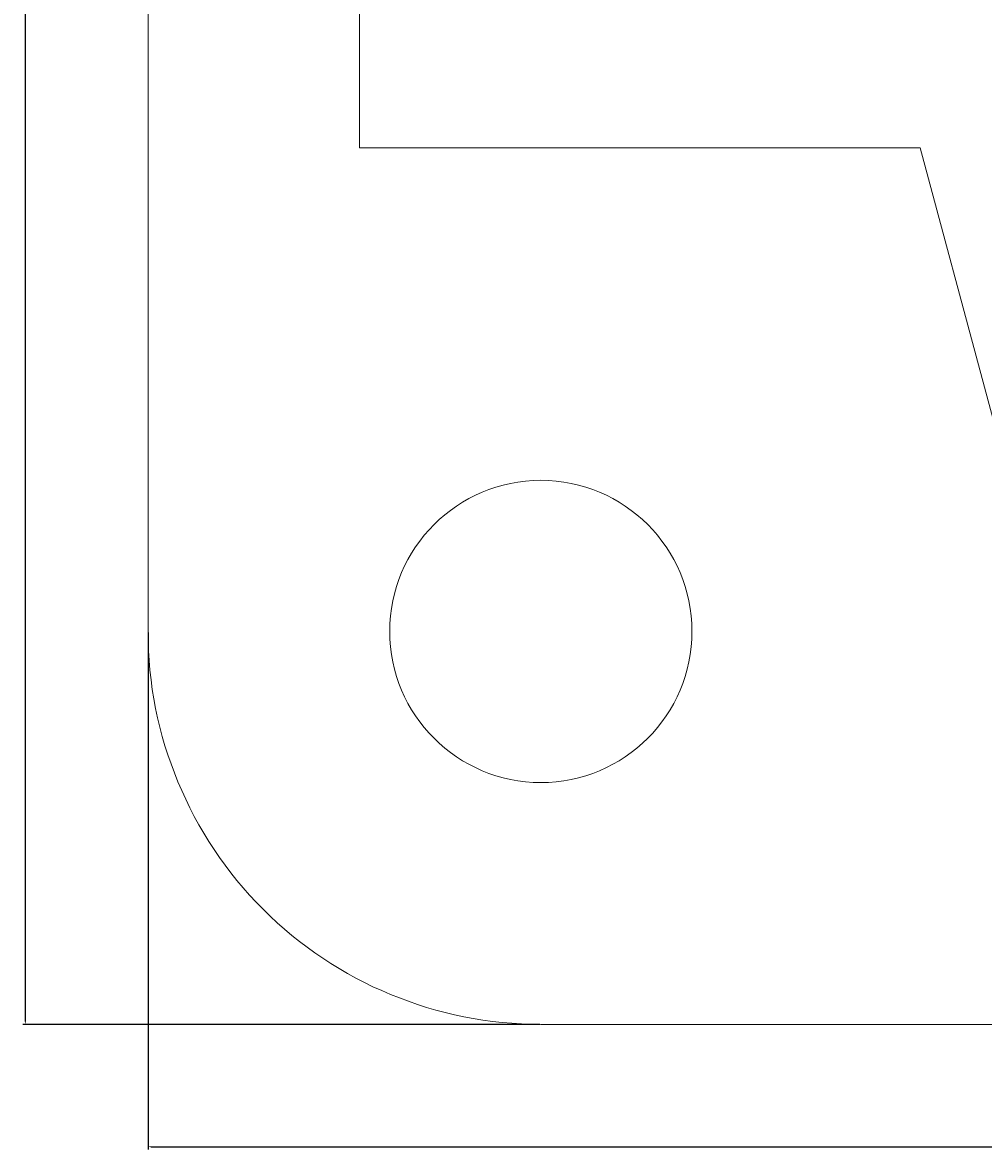
# Model space of a CAD drawing. Units: millimetres. Extents: x 2597 to 2768, y 1809 to 1980.
# Tile 1 of 7: x 2597 to 2661, y 1809 to 1884. Entities that reach past the tile are written whole.
import ezdxf

# ---------------------------------------------------------------- set-up
doc = ezdxf.new("R2010")
doc.units = ezdxf.units.MM
doc.layers.add('M-CONS', color=8, linetype='Continuous', lineweight=18)
doc.layers.add('M-DIMS', color=2, linetype='Continuous', lineweight=18)
doc.styles.get("Standard").update_dxf_attribs({"font": 'arial.ttf'})
doc.dimstyles.get("Standard").update_dxf_attribs({"dimtxt": 0.18, "dimasz": 0.18, "dimexe": 0.18, "dimexo": 0.0625, "dimgap": 0.09, "dimtad": 0, "dimtih": 1, "dimtoh": 1, "dimdec": 4, "dimzin": 0, "dimdsep": 46, "dimtxsty": 'Standard', "dimcen": 0.09, "dimadec": 0, "dimazin": 0, "dimtfac": 1, "dimtdec": 4, "dimtofl": 0, "dimtmove": 0, "dimatfit": 3, "dimfxl": 1, "dimtolj": 1, "dimtzin": 0, "dimarcsym": 0})

# ---------------------------------------------------------------- blocks, each defined once
blk = doc.blocks.new('*D3')
at = {"layer": 'Defpoints', "color": 0, "transparency": 16777216}
for p in [(2605.776, 1843.43), (2759.776, 1843.43), (2759.776, 1809.33)]:
    blk.add_point(p, dxfattribs=at)
at = {"layer": 'M-DIMS', "color": 0, "lineweight": -2, "transparency": 16777216}
for p, q in [((2605.776, 1843.368), (2605.776, 1809.15)), ((2759.776, 1843.368), (2759.776, 1809.15)), ((2605.956, 1809.33), (2682.496, 1809.33)), ((2759.596, 1809.33), (2683.056, 1809.33))]:
    blk.add_line(p, q, dxfattribs=at)
at = {"layer": 'M-DIMS', "color": 0, "transparency": 16777216}
for points in [[(2605.956, 1809.36), (2605.956, 1809.3), (2605.776, 1809.33)], [(2759.596, 1809.36), (2759.596, 1809.3), (2759.776, 1809.33)]]:
    blk.add_solid(points, dxfattribs=at)
at = {"layer": 'M-DIMS', "color": 0, "transparency": 16777216, "insert": (2682.776, 1809.33), "char_height": 0.18, "attachment_point": 5}
blk.add_mtext('\\A1;154', dxfattribs=at)
blk = doc.blocks.new('*D4')
at = {"layer": 'Defpoints', "color": 0, "transparency": 16777216}
for p in [(2597.676, 1971.43), (2631.776, 1971.43), (2631.776, 1817.43)]:
    blk.add_point(p, dxfattribs=at)
at = {"layer": 'M-DIMS', "color": 0, "lineweight": -2, "transparency": 16777216}
for p, q in [((2631.713, 1971.43), (2597.496, 1971.43)), ((2597.676, 1971.25), (2597.676, 1894.612)), ((2597.676, 1817.61), (2597.676, 1894.248)), ((2631.713, 1817.43), (2597.496, 1817.43))]:
    blk.add_line(p, q, dxfattribs=at)
at = {"layer": 'M-DIMS', "color": 0, "transparency": 16777216}
for points in [[(2597.646, 1971.25), (2597.706, 1971.25), (2597.676, 1971.43)], [(2597.646, 1817.61), (2597.706, 1817.61), (2597.676, 1817.43)]]:
    blk.add_solid(points, dxfattribs=at)
at = {"layer": 'M-DIMS', "color": 0, "transparency": 16777216, "insert": (2597.676, 1894.43), "char_height": 0.18, "attachment_point": 5}
blk.add_mtext('\\A1;154', dxfattribs=at)

msp = doc.modelspace()

# ---------------------------------------------------------------- linework, layer by layer
at = {"layer": 'M-CONS', "extrusion": (0, -1, 0)}
msp.add_line((2656.8814, 1875.4301, 56), (2636.8814, 1875.4301, 56), dxfattribs=at)
at = {"layer": 'M-CONS'}
msp.add_lwpolyline([(2631.7756, 1817.4301), (2733.7756, 1817.4301, 0.4142136), (2759.7756, 1843.4301), (2759.7756, 1945.4301, 0.4142136), (2733.7756, 1971.4301), (2631.7756, 1971.4301, 0.4142136), (2605.7756, 1945.4301), (2605.7756, 1843.4301, 0.4142136)], format="xyb", close=True, dxfattribs=at)
msp.add_lwpolyline([(2713.7756, 1903.4301), (2745.7756, 1903.4301), (2745.7756, 1913.4301), (2708.6698, 1913.4301), (2700.1588, 1945.1014, 0.7667514), (2665.3923, 1945.1014), (2656.8814, 1913.4301), (2619.7756, 1913.4301), (2619.7756, 1903.4301), (2651.7756, 1903.4301), (2651.7756, 1885.4301), (2619.7756, 1885.4301), (2619.7756, 1875.4301), (2656.8814, 1875.4301), (2665.3923, 1843.7587, 0.7667514), (2700.1588, 1843.7587), (2708.6698, 1875.4301), (2745.7756, 1875.4301), (2745.7756, 1885.4301), (2713.7756, 1885.4301), (2713.7756, 1903.4301), (2713.7756, 1894.4301)], format="xyb", dxfattribs=at)
at = {"layer": 'M-CONS', "extrusion": (0, -1, 0)}
msp.add_circle((2636.8814, 44, -1875.4301), 5, dxfattribs=at)
at = {"layer": 'M-CONS'}
msp.add_circle((2631.7756, 1843.4301), 10, dxfattribs=at)

# ---------------------------------------------------------------- dimensions: what is measured, and where the dimension line sits
at = {"layer": 'M-DIMS'}
dim = msp.add_linear_dim(base=(2597.6756, 1971.4301), p1=(2631.7756, 1817.4301), p2=(2631.7756, 1971.4301), angle=90, dimstyle='Standard', override={"dimdec": 0, "dimlfac": 1, "dimrnd": 0, "dimzin": 0, "dimdsep": 46, "dimlunit": 2}, dxfattribs=at)
dim.commit()
dim.dimension.update_dxf_attribs({"geometry": '*D4', "text_midpoint": (2597.6756, 1894.4301)})
dim = msp.add_linear_dim(base=(2759.7756, 1809.3301), p1=(2605.7756, 1843.4301), p2=(2759.7756, 1843.4301), dimstyle='Standard', override={"dimdec": 0, "dimlfac": 1, "dimrnd": 0, "dimzin": 0, "dimdsep": 46, "dimlunit": 2}, dxfattribs=at)
dim.commit()
dim.dimension.update_dxf_attribs({"geometry": '*D3', "text_midpoint": (2682.7756, 1809.3301)})

doc.saveas('drawing.dxf')
